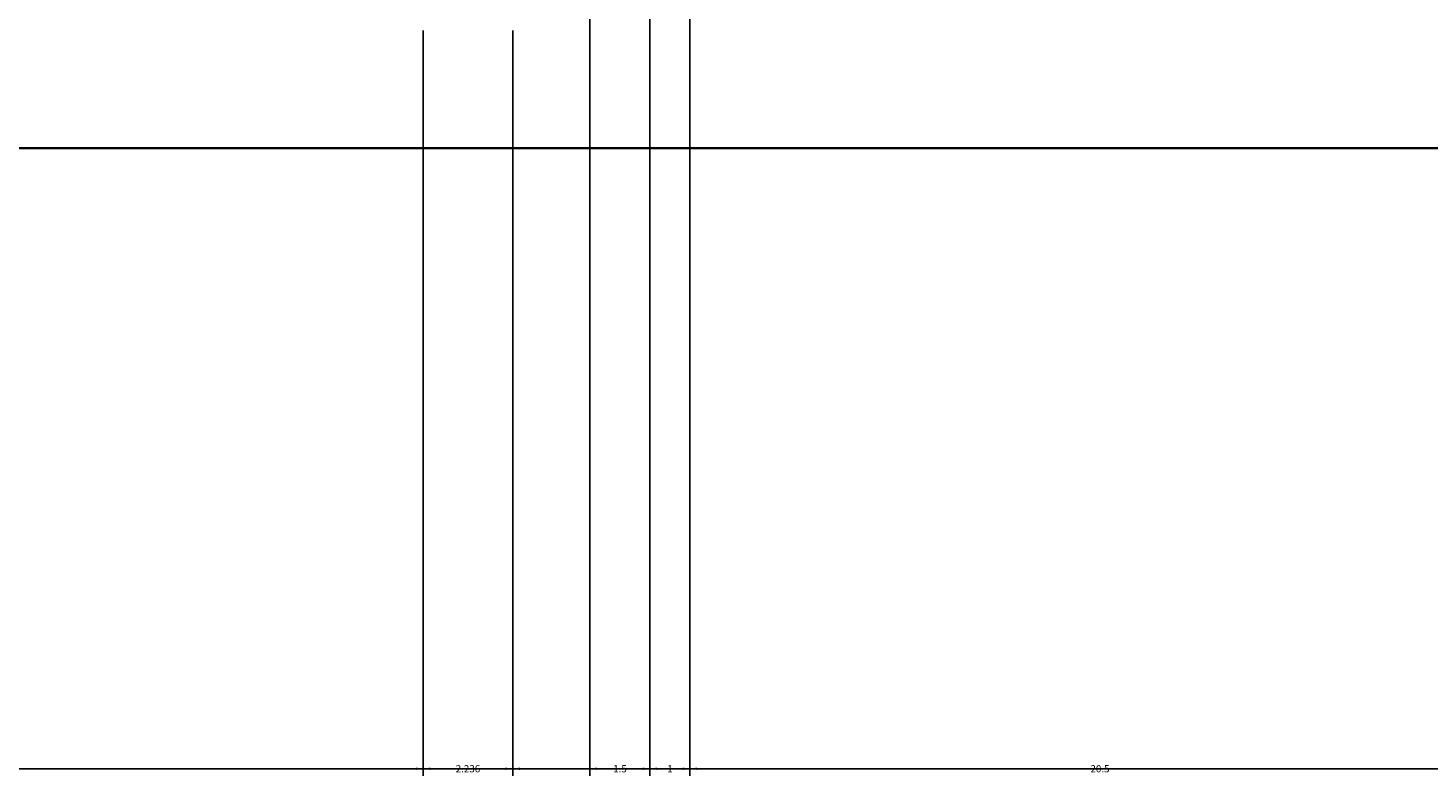
# Model space of a CAD drawing. Units: inches. Extents: x -6 to 289, y -8 to 323.
# Tile 28 of 107: x 174 to 209, y -8 to 10. Entities that reach past the tile are written whole.
import ezdxf

# ---------------------------------------------------------------- set-up
doc = ezdxf.new("R2010")
doc.units = ezdxf.units.IN
doc.header["$MEASUREMENT"] = 0
for name, color, linetype, lineweight in [('A-ANNO-DIMS', 2, 'Continuous', 18), ('A-DOOR', 3, 'Continuous', 25), ('A-ELEV', 7, 'Continuous', 35)]:
    doc.layers.add(name, color=color, linetype=linetype, lineweight=lineweight)
doc.styles.get("Standard").update_dxf_attribs({"font": 'arial.ttf'})
doc.dimstyles.get("Standard").update_dxf_attribs({"dimtxt": 0.18, "dimasz": 0.18, "dimexe": 0.18, "dimexo": 0.0625, "dimgap": 0.09, "dimtad": 0, "dimtih": 1, "dimtoh": 1, "dimdec": 4, "dimzin": 0, "dimdsep": 46, "dimtxsty": 'Standard', "dimcen": 0.09, "dimadec": 0, "dimazin": 0, "dimtfac": 1, "dimtdec": 4, "dimtofl": 0, "dimtmove": 0, "dimatfit": 3, "dimfxl": 1, "dimtolj": 1, "dimtzin": 0, "dimarcsym": 0})

# ---------------------------------------------------------------- blocks, each defined once
blk = doc.blocks.new('*D16')
at = {"layer": 'A-ANNO-DIMS', "color": 0, "lineweight": -2, "transparency": 16777216}
for p, q in [((9.943, 68.37), (9.943, -8.391)), ((272.973, 68.37), (272.973, -8.391)), ((10.123, -8.211), (140.993, -8.211)), ((272.793, -8.211), (141.923, -8.211))]:
    blk.add_line(p, q, dxfattribs=at)
at = {"layer": 'A-ANNO-DIMS', "color": 0, "transparency": 16777216}
for points in [[(10.123, -8.181), (10.123, -8.241), (9.943, -8.211)], [(272.793, -8.181), (272.793, -8.241), (272.973, -8.211)]]:
    blk.add_solid(points, dxfattribs=at)
at = {"layer": 'Defpoints', "color": 0, "transparency": 16777216}
for p in [(9.943, 68.432), (272.973, 68.432), (272.973, -8.211)]:
    blk.add_point(p, dxfattribs=at)
at = {"layer": 'A-ANNO-DIMS', "color": 0, "transparency": 16777216, "insert": (141.458, -8.211), "char_height": 0.18, "attachment_point": 5}
blk.add_mtext('\\A1;263.03', dxfattribs=at)
blk = doc.blocks.new('*D40')
at = {"layer": 'A-ANNO-DIMS', "color": 0, "lineweight": -2, "transparency": 16777216}
for p, q in [((188.292, 226.826), (188.292, -8.391)), ((189.792, 225.326), (189.792, -8.391)), ((188.472, -8.211), (188.796, -8.211)), ((189.612, -8.211), (189.288, -8.211))]:
    blk.add_line(p, q, dxfattribs=at)
at = {"layer": 'A-ANNO-DIMS', "color": 0, "transparency": 16777216}
for points in [[(188.472, -8.181), (188.472, -8.241), (188.292, -8.211)], [(189.612, -8.181), (189.612, -8.241), (189.792, -8.211)]]:
    blk.add_solid(points, dxfattribs=at)
at = {"layer": 'Defpoints', "color": 0, "transparency": 16777216}
for p in [(188.292, 226.889), (189.792, 225.389), (189.792, -8.211)]:
    blk.add_point(p, dxfattribs=at)
at = {"layer": 'A-ANNO-DIMS', "color": 0, "transparency": 16777216, "insert": (189.042, -8.211), "char_height": 0.18, "attachment_point": 5}
blk.add_mtext('\\A1;1.5', dxfattribs=at)
blk = doc.blocks.new('*D41')
at = {"layer": 'A-ANNO-DIMS', "color": 0, "lineweight": -2, "transparency": 16777216}
for p, q in [((189.792, 225.326), (189.792, -8.391)), ((190.792, 224.326), (190.792, -8.391)), ((189.972, -8.211), (190.169, -8.211)), ((190.612, -8.211), (190.415, -8.211))]:
    blk.add_line(p, q, dxfattribs=at)
at = {"layer": 'A-ANNO-DIMS', "color": 0, "transparency": 16777216}
for points in [[(189.972, -8.181), (189.972, -8.241), (189.792, -8.211)], [(190.612, -8.181), (190.612, -8.241), (190.792, -8.211)]]:
    blk.add_solid(points, dxfattribs=at)
at = {"layer": 'Defpoints', "color": 0, "transparency": 16777216}
for p in [(189.792, 225.389), (190.792, 224.389), (190.792, -8.211)]:
    blk.add_point(p, dxfattribs=at)
at = {"layer": 'A-ANNO-DIMS', "color": 0, "transparency": 16777216, "insert": (190.292, -8.211), "char_height": 0.18, "attachment_point": 5}
blk.add_mtext('\\A1;1', dxfattribs=at)
blk = doc.blocks.new('*D42')
at = {"layer": 'A-ANNO-DIMS', "color": 0, "lineweight": -2, "transparency": 16777216}
for p, q in [((190.792, 224.326), (190.792, -8.391)), ((211.292, 224.326), (211.292, -8.391)), ((190.972, -8.211), (200.716, -8.211)), ((211.112, -8.211), (201.368, -8.211))]:
    blk.add_line(p, q, dxfattribs=at)
at = {"layer": 'A-ANNO-DIMS', "color": 0, "transparency": 16777216}
for points in [[(190.972, -8.181), (190.972, -8.241), (190.792, -8.211)], [(211.112, -8.181), (211.112, -8.241), (211.292, -8.211)]]:
    blk.add_solid(points, dxfattribs=at)
at = {"layer": 'Defpoints', "color": 0, "transparency": 16777216}
for p in [(190.792, 224.389), (211.292, 224.389), (211.292, -8.211)]:
    blk.add_point(p, dxfattribs=at)
at = {"layer": 'A-ANNO-DIMS', "color": 0, "transparency": 16777216, "insert": (201.042, -8.211), "char_height": 0.18, "attachment_point": 5}
blk.add_mtext('\\A1;20.5', dxfattribs=at)
blk = doc.blocks.new('*D68')
at = {"layer": 'A-ANNO-DIMS', "color": 0, "lineweight": -2, "transparency": 16777216}
for p, q in [((124.008, 10.226), (124.008, -8.391)), ((184.124, 10.226), (184.124, -8.391)), ((124.188, -8.211), (153.673, -8.211)), ((183.944, -8.211), (154.459, -8.211))]:
    blk.add_line(p, q, dxfattribs=at)
at = {"layer": 'A-ANNO-DIMS', "color": 0, "transparency": 16777216}
for points in [[(124.188, -8.181), (124.188, -8.241), (124.008, -8.211)], [(183.944, -8.181), (183.944, -8.241), (184.124, -8.211)]]:
    blk.add_solid(points, dxfattribs=at)
at = {"layer": 'Defpoints', "color": 0, "transparency": 16777216}
for p in [(124.008, 10.289), (184.124, 10.289), (184.124, -8.211)]:
    blk.add_point(p, dxfattribs=at)
at = {"layer": 'A-ANNO-DIMS', "color": 0, "transparency": 16777216, "insert": (154.066, -8.211), "char_height": 0.18, "attachment_point": 5}
blk.add_mtext('\\A1;60.12', dxfattribs=at)
blk = doc.blocks.new('*D69')
at = {"layer": 'A-ANNO-DIMS', "color": 0, "lineweight": -2, "transparency": 16777216}
for p, q in [((184.124, 10.226), (184.124, -8.391)), ((186.36, 10.226), (186.36, -8.391)), ((184.304, -8.211), (184.847, -8.211)), ((186.18, -8.211), (185.638, -8.211))]:
    blk.add_line(p, q, dxfattribs=at)
at = {"layer": 'A-ANNO-DIMS', "color": 0, "transparency": 16777216}
for points in [[(184.304, -8.181), (184.304, -8.241), (184.124, -8.211)], [(186.18, -8.181), (186.18, -8.241), (186.36, -8.211)]]:
    blk.add_solid(points, dxfattribs=at)
at = {"layer": 'Defpoints', "color": 0, "transparency": 16777216}
for p in [(184.124, 10.289), (186.36, 10.289), (186.36, -8.211)]:
    blk.add_point(p, dxfattribs=at)
at = {"layer": 'A-ANNO-DIMS', "color": 0, "transparency": 16777216, "insert": (185.242, -8.211), "char_height": 0.18, "attachment_point": 5}
blk.add_mtext('\\A1;2.236', dxfattribs=at)
blk = doc.blocks.new('*D70')
at = {"layer": 'A-ANNO-DIMS', "color": 0, "lineweight": -2, "transparency": 16777216}
for p, q in [((186.36, 10.226), (186.36, -8.391)), ((244.241, 10.226), (244.241, -8.391)), ((186.54, -8.211), (214.907, -8.211)), ((244.061, -8.211), (215.694, -8.211))]:
    blk.add_line(p, q, dxfattribs=at)
at = {"layer": 'A-ANNO-DIMS', "color": 0, "transparency": 16777216}
for points in [[(186.54, -8.181), (186.54, -8.241), (186.36, -8.211)], [(244.061, -8.181), (244.061, -8.241), (244.241, -8.211)]]:
    blk.add_solid(points, dxfattribs=at)
at = {"layer": 'Defpoints', "color": 0, "transparency": 16777216}
for p in [(186.36, 10.289), (244.241, 10.289), (244.241, -8.211)]:
    blk.add_point(p, dxfattribs=at)
at = {"layer": 'A-ANNO-DIMS', "color": 0, "transparency": 16777216, "insert": (215.301, -8.211), "char_height": 0.18, "attachment_point": 5}
blk.add_mtext('\\A1;57.88', dxfattribs=at)

msp = doc.modelspace()

# ---------------------------------------------------------------- linework, layer by layer
at = {"layer": 'A-DOOR'}
msp.add_lwpolyline([(121.008, 51.0851), (247.2408, 51.0851), (247.2408, 7.2888), (121.008, 7.2888)], close=True, dxfattribs=at)
at = {"layer": 'A-ELEV'}
msp.add_line((19.1638, 7.2888), (271.1638, 7.2888), dxfattribs=at)

# ---------------------------------------------------------------- dimensions: what is measured, and where the dimension line sits
at = {"layer": 'A-ANNO-DIMS'}
for base, p1, p2, override, picture, middle in [((189.7918, -8.2112), (188.2918, 226.8887), (189.7918, 225.3887), {"dimdec": 1, "dimlfac": 1, "dimrnd": 0, "dimzin": 0, "dimdsep": 46, "dimlunit": 2}, '*D40', (189.0418, -8.2112)), ((190.7918, -8.2112), (189.7918, 225.3887), (190.7918, 224.3887), {"dimdec": 0, "dimlfac": 1, "dimrnd": 0, "dimzin": 0, "dimdsep": 46, "dimlunit": 2}, '*D41', (190.2918, -8.2112)), ((211.2918, -8.2112), (190.7918, 224.3887), (211.2918, 224.3887), {"dimdec": 1, "dimlfac": 1, "dimrnd": 0, "dimzin": 0, "dimdsep": 46, "dimlunit": 2}, '*D42', (201.0418, -8.2112)), ((272.9733, -8.2112), (9.943, 68.4322), (272.9733, 68.4322), {"dimdec": 2, "dimlfac": 1, "dimrnd": 0, "dimzin": 0, "dimdsep": 46, "dimlunit": 2}, '*D16', (141.4581, -8.2112)), ((184.1244, -8.2112), (124.008, 10.2888), (184.1244, 10.2888), {"dimdec": 2, "dimlfac": 1, "dimrnd": 0, "dimzin": 0, "dimdsep": 46, "dimlunit": 2}, '*D68', (154.0662, -8.2112)), ((186.3604, -8.2112), (184.1244, 10.2888), (186.3604, 10.2888), {"dimdec": 3, "dimlfac": 1, "dimrnd": 0, "dimzin": 0, "dimdsep": 46, "dimlunit": 2}, '*D69', (185.2424, -8.2112)), ((244.2408, -8.2112), (186.3604, 10.2888), (244.2408, 10.2888), {"dimdec": 2, "dimlfac": 1, "dimrnd": 0, "dimzin": 0, "dimdsep": 46, "dimlunit": 2}, '*D70', (215.3006, -8.2112))]:
    dim = msp.add_linear_dim(base=base, p1=p1, p2=p2, dimstyle='Standard', override=override, dxfattribs=at)
    dim.commit()
    dim.dimension.update_dxf_attribs({"geometry": picture, "text_midpoint": middle})

doc.saveas('drawing.dxf')
